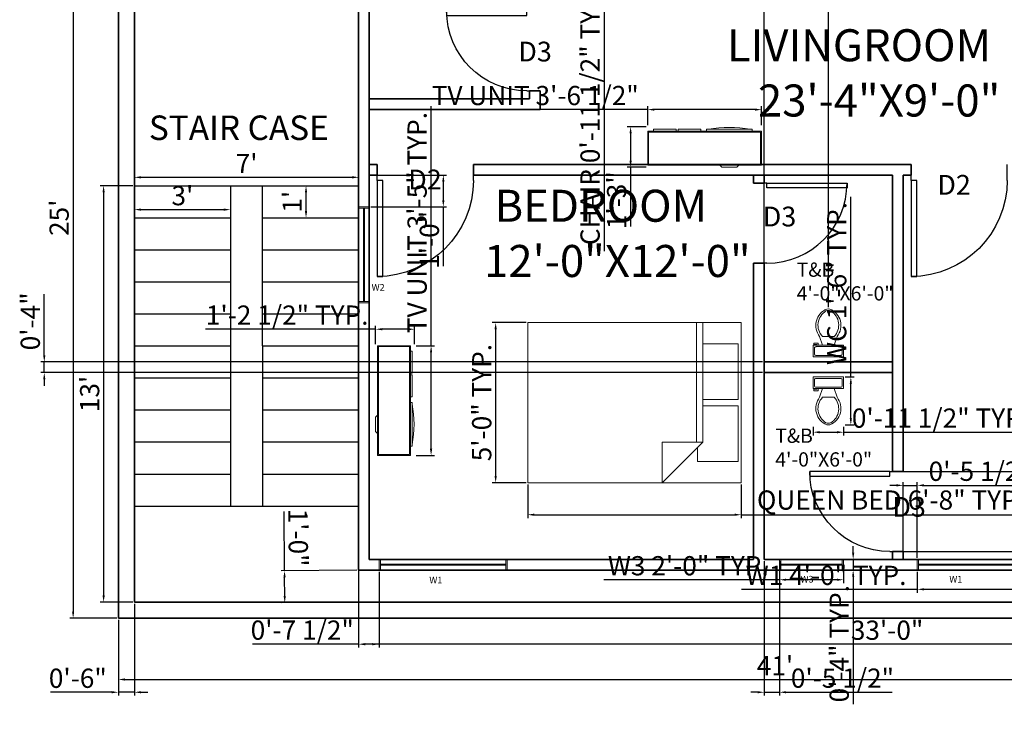
# Model space of a CAD drawing. Units: inches. Extents: x 2165 to 6441, y 2023 to 4425.
# Tile 1 of 4: x 2165 to 2534, y 2023 to 2281. Entities that reach past the tile are written whole.
import ezdxf

# ---------------------------------------------------------------- set-up
doc = ezdxf.new("R2010")
doc.units = ezdxf.units.IN
for name, color, linetype, lineweight in [('A-ANNO-DIMS', 7, 'Continuous', 18), ('A-ANNO-TEXT', 1, 'Continuous', 18), ('A-AREA-IDEN', 1, 'Continuous', 25), ('A-FLOR-FIXT', 9, 'Continuous', 18), ('C-PROP', 7, 'Continuous', 35), ('doors', 5, 'Continuous', 25), ('furniture', 9, 'Continuous', 18), ('stair case', 6, 'Continuous', 25), ('walls', 7, 'Continuous', 35), ('windows', 72, 'Continuous', 18)]:
    doc.layers.add(name, color=color, linetype=linetype, lineweight=lineweight)
doc.styles.get("Standard").update_dxf_attribs({"font": 'arial.ttf'})
doc.dimstyles.new('ISO-25', dxfattribs={"dimtxt": 7.203125, "dimasz": 2.5, "dimexe": 1.25, "dimexo": 0.625, "dimtad": 1, "dimdec": 0, "dimlunit": 4, "dimtxsty": 'Standard', "dimcen": 2.5, "dimadec": 0, "dimazin": 0, "dimtfac": 1, "dimtdec": 0, "dimtmove": 0, "dimatfit": 3, "dimfxl": 1, "dimarcsym": 0})

# ---------------------------------------------------------------- blocks, each defined once
blk = doc.blocks.new('*U2')
for p, q in [((0, 0), (0, -5)), ((30, 0), (30, -5))]:
    blk.add_line(p, q)
blk.add_lwpolyline([(0, 0), (0, 30), (1.75, 30), (1.75, 0)], close=True)
blk.add_arc((0, 0), 30, 0, 90)
blk = doc.blocks.new('Bed - Queen')
for p, q in [((0, -80.00003), (0, 0)), ((0, 0), (59.99999, 0)), ((59.99999, 0), (59.99999, -80.00003)), ((7.99999, -1.2), (28.79998, -1.2)), ((7.99999, -14.4), (7.99999, -1.2)), ((28.79998, -1.2), (28.79998, -14.4)), ((31.19999, -1.2), (51.99999, -1.2)), ((31.19999, -14.4), (31.19999, -1.2)), ((51.99999, -1.2), (51.99999, -16.4)), ((0, -14.4), (44.8, -14.4)), ((59.99999, -29.6), (44.8, -14.4)), ((44.8, -14.4), (44.8, -29.6)), ((44.8, -16.8), (0, -16.8)), ((51.99999, -16.4), (46.79936, -16.4)), ((44.8, -29.6), (59.99999, -29.6)), ((59.99999, -80.00003), (0, -80.00003))]:
    blk.add_line(p, q)
blk = doc.blocks.new('Entertainment Center')
for p, q in [((-4, 0), (-5, -1)), ((4, 0), (-4, 0)), ((5, -1), (4, 0)), ((-17, -19), (-17, -1)), ((-17, -1), (43, -1)), ((-16.5, -18.5), (-16.5, -1.5)), ((-16.5, -1.5), (42.5, -1.5)), ((42.5, -1.5), (42.5, -18.5)), ((43, -1), (43, -19)), ((43, -19), (-17, -19)), ((42.5, -18.5), (-16.5, -18.5)), ((-12, -20), (-12, -19)), ((12, -20), (-12, -20)), ((12, -19), (12, -20)), ((15, -20), (15, -19)), ((27, -20), (15, -20)), ((27, -19), (27, -20)), ((28, -20), (28, -19)), ((40, -20), (28, -20)), ((40, -19), (40, -20))]:
    blk.add_line(p, q)
blk.add_arc((0, 40), 61, 259.6111, 280.3889)
blk = doc.blocks.new('Toilet - top')
for p, q in [((9.5, -6), (9.5, -2)), ((-10, -8.5), (-8, -8.5)), ((-10, -9.5), (-10, -8.5)), ((-7, -9.5), (-10, -9.5)), ((-8, -8.5), (-8, -8)), ((-7, -8), (-7, -9.5)), ((-4, -8), (-6, -14)), ((4, -8), (6, -14)), ((4, -14), (-4, -14))]:
    blk.add_line(p, q)
blk.add_lwpolyline([(10.5, -8), (10.5, 0), (-10.5, 0), (-10.5, -8)], close=True)
for points in [[(-9.5, -2), (-9.5, -6)], [(8.5, -1), (-8.5, -1)], [(-8.5, -7), (8.5, -7)]]:
    blk.add_lwpolyline(points)
for centre, radius, start, end in [((-8.62, -1.88), 0.884, 81.8699, 188.1301), ((-8.62, -6.12), 0.884, 171.8699, 278.1301), ((8.62, -1.88), 0.884, 351.8699, 98.1301), ((8.62, -6.12), 0.884, 261.8699, 8.1301), ((3.52, -21.58), 12.17, 141.46911, 247.97143), ((4.2, -21.82), 11.33, 136.36773, 238.94682), ((-3.52, -21.58), 12.17, 292.02843, 38.53071), ((-4.2, -21.82), 11.33, 301.05301, 43.63209), ((0, -27.88), 4, 245.73182, 294.26817), ((0, -29), 4, 254.86053, 285.13947)]:
    blk.add_arc(centre, radius, start, end)
blk = doc.blocks.new('*D10')
at = {"layer": 'A-ANNO-DIMS', "color": 0, "lineweight": -2, "transparency": 16777216}
for p, q in [((2201.06, 2356.78), (2183.49, 2356.78)), ((2184.74, 2354.28), (2184.74, 2059.28)), ((2201.06, 2056.78), (2183.49, 2056.78))]:
    blk.add_line(p, q, dxfattribs=at)
at = {"layer": 'A-ANNO-DIMS', "color": 0, "transparency": 16777216}
for points in [[(2184.32, 2354.28), (2185.15, 2354.28), (2184.74, 2356.78)], [(2184.32, 2059.28), (2185.15, 2059.28), (2184.74, 2056.78)]]:
    blk.add_solid(points, dxfattribs=at)
at = {"layer": 'Defpoints', "color": 0, "transparency": 16777216}
for p in [(2201.68, 2356.78), (2184.74, 2056.78), (2201.68, 2056.78)]:
    blk.add_point(p, dxfattribs=at)
at = {"layer": 'A-ANNO-DIMS', "color": 0, "transparency": 16777216, "insert": (2180.43, 2206.78), "char_height": 7.203, "attachment_point": 5, "rotation": 90}
blk.add_mtext("25'", dxfattribs=at)
blk = doc.blocks.new('*D11')
at = {"layer": 'A-ANNO-DIMS', "color": 0, "lineweight": -2, "transparency": 16777216}
for p, q in [((2201.68, 2056.16), (2201.68, 2032.56)), ((2693.68, 2056.16), (2693.68, 2032.56)), ((2204.18, 2033.81), (2691.18, 2033.81))]:
    blk.add_line(p, q, dxfattribs=at)
at = {"layer": 'A-ANNO-DIMS', "color": 0, "transparency": 16777216}
for points in [[(2204.18, 2034.23), (2204.18, 2033.39), (2201.68, 2033.81)], [(2691.18, 2034.23), (2691.18, 2033.39), (2693.68, 2033.81)]]:
    blk.add_solid(points, dxfattribs=at)
at = {"layer": 'Defpoints', "color": 0, "transparency": 16777216}
for p in [(2201.68, 2056.78), (2693.68, 2056.78), (2693.68, 2033.81)]:
    blk.add_point(p, dxfattribs=at)
at = {"layer": 'A-ANNO-DIMS', "color": 0, "transparency": 16777216, "insert": (2447.68, 2038.05), "char_height": 7.203, "attachment_point": 5}
blk.add_mtext("41'", dxfattribs=at)
blk = doc.blocks.new('*D12')
at = {"layer": 'A-ANNO-DIMS', "color": 0, "lineweight": -2, "transparency": 16777216}
for p, q in [((2207.68, 2218.16), (2207.68, 2208.58)), ((2243.68, 2218.16), (2243.68, 2208.58)), ((2210.18, 2209.83), (2241.18, 2209.83))]:
    blk.add_line(p, q, dxfattribs=at)
at = {"layer": 'A-ANNO-DIMS', "color": 0, "transparency": 16777216}
for points in [[(2210.18, 2210.25), (2210.18, 2209.41), (2207.68, 2209.83)], [(2241.18, 2210.25), (2241.18, 2209.41), (2243.68, 2209.83)]]:
    blk.add_solid(points, dxfattribs=at)
at = {"layer": 'Defpoints', "color": 0, "transparency": 16777216}
for p in [(2207.68, 2218.78), (2243.68, 2218.78), (2243.68, 2209.83)]:
    blk.add_point(p, dxfattribs=at)
at = {"layer": 'A-ANNO-DIMS', "color": 0, "transparency": 16777216, "insert": (2225.68, 2214.13), "char_height": 7.203, "attachment_point": 5}
blk.add_mtext("3'", dxfattribs=at)
blk = doc.blocks.new('*D13')
at = {"layer": 'A-ANNO-DIMS', "color": 0, "lineweight": -2, "transparency": 16777216}
for p, q in [((2256.31, 2218.78), (2273.24, 2218.78)), ((2271.99, 2209.28), (2271.99, 2216.28)), ((2256.32, 2206.78), (2273.24, 2206.78))]:
    blk.add_line(p, q, dxfattribs=at)
at = {"layer": 'A-ANNO-DIMS', "color": 0, "transparency": 16777216}
for points in [[(2271.58, 2216.28), (2272.41, 2216.28), (2271.99, 2218.78)], [(2271.58, 2209.28), (2272.41, 2209.28), (2271.99, 2206.78)]]:
    blk.add_solid(points, dxfattribs=at)
at = {"layer": 'Defpoints', "color": 0, "transparency": 16777216}
for p in [(2255.69, 2218.78), (2271.99, 2218.78), (2255.69, 2206.78)]:
    blk.add_point(p, dxfattribs=at)
at = {"layer": 'A-ANNO-DIMS', "color": 0, "transparency": 16777216, "insert": (2267.75, 2212.78), "char_height": 7.203, "attachment_point": 5, "rotation": 90}
blk.add_mtext("1'", dxfattribs=at)
blk = doc.blocks.new('*D14')
at = {"layer": 'A-ANNO-DIMS', "color": 0, "lineweight": -2, "transparency": 16777216}
for p, q in [((2207.68, 2219.41), (2207.68, 2223.18)), ((2210.18, 2221.93), (2289.28, 2221.93)), ((2291.78, 2219.41), (2291.78, 2223.18))]:
    blk.add_line(p, q, dxfattribs=at)
at = {"layer": 'A-ANNO-DIMS', "color": 0, "transparency": 16777216}
for points in [[(2210.18, 2222.35), (2210.18, 2221.52), (2207.68, 2221.93)], [(2289.28, 2222.35), (2289.28, 2221.52), (2291.78, 2221.93)]]:
    blk.add_solid(points, dxfattribs=at)
at = {"layer": 'Defpoints', "color": 0, "transparency": 16777216}
for p in [(2291.78, 2221.93), (2207.68, 2218.78), (2291.78, 2218.78)]:
    blk.add_point(p, dxfattribs=at)
at = {"layer": 'A-ANNO-DIMS', "color": 0, "transparency": 16777216, "insert": (2249.73, 2226.16), "char_height": 7.203, "attachment_point": 5}
blk.add_mtext("7'", dxfattribs=at)
blk = doc.blocks.new('*D22')
at = {"layer": 'A-ANNO-DIMS', "color": 0, "lineweight": -2, "transparency": 16777216}
for p, q in [((2207.06, 2218.78), (2194.91, 2218.78)), ((2196.16, 2216.28), (2196.16, 2065.28)), ((2207.06, 2062.78), (2194.91, 2062.78))]:
    blk.add_line(p, q, dxfattribs=at)
at = {"layer": 'A-ANNO-DIMS', "color": 0, "transparency": 16777216}
for points in [[(2195.75, 2216.28), (2196.58, 2216.28), (2196.16, 2218.78)], [(2195.75, 2065.28), (2196.58, 2065.28), (2196.16, 2062.78)]]:
    blk.add_solid(points, dxfattribs=at)
at = {"layer": 'Defpoints', "color": 0, "transparency": 16777216}
for p in [(2207.68, 2218.78), (2196.16, 2062.78), (2207.68, 2062.78)]:
    blk.add_point(p, dxfattribs=at)
at = {"layer": 'A-ANNO-DIMS', "color": 0, "transparency": 16777216, "insert": (2191.86, 2140.78), "char_height": 7.203, "attachment_point": 5, "rotation": 90}
blk.add_mtext("13'", dxfattribs=at)
blk = doc.blocks.new('WIN-W2-36IN')
for p, q in [((0, 4), (36, 4)), ((0, 0), (0, 4)), ((0.5, 0), (0.5, 4)), ((35.5, 4), (35.5, 0)), ((36, 4), (36, 0)), ((36, 0), (0, 0)), ((0.5, 2.2), (35.5, 2.2)), ((0.5, 1.8), (35.5, 1.8)), ((0.5, 1.8), (35.5, 1.8))]:
    blk.add_line(p, q)
blk = doc.blocks.new('WIN-W1-48IN')
for p, q in [((0, 4), (48, 4)), ((0, 0), (0, 4)), ((0.5, 0), (0.5, 4)), ((47.5, 4), (47.5, 0)), ((48, 4), (48, 0)), ((48, 0), (0, 0)), ((0.5, 2.2), (47.5, 2.2)), ((0.5, 1.8), (47.5, 1.8))]:
    blk.add_line(p, q)
blk = doc.blocks.new('WIN-W3-24IN')
for p, q in [((0, 4), (24, 4)), ((0, 0), (0, 4)), ((0.5, 0), (0.5, 4)), ((23.5, 0), (23.5, 4)), ((24, 0), (24, 4)), ((24, 0), (0, 0)), ((23.5, 2.2), (0.5, 2.2)), ((23.5, 1.8), (0.5, 1.8))]:
    blk.add_line(p, q)
blk = doc.blocks.new('*D26')
at = {"layer": 'A-ANNO-DIMS', "color": 0, "lineweight": -2, "transparency": 16777216}
for p, q in [((2500.99, 2074.16), (2500.99, 2066.33)), ((2549, 2074.16), (2549, 2066.33)), ((2500.99, 2067.58), (2435.15, 2067.58)), ((2546.5, 2067.58), (2503.49, 2067.58))]:
    blk.add_line(p, q, dxfattribs=at)
at = {"layer": 'A-ANNO-DIMS', "color": 0, "transparency": 16777216}
for points in [[(2503.49, 2068), (2503.49, 2067.17), (2500.99, 2067.58)], [(2546.5, 2068), (2546.5, 2067.17), (2549, 2067.58)]]:
    blk.add_solid(points, dxfattribs=at)
at = {"layer": 'Defpoints', "color": 0, "transparency": 16777216}
for p in [(2500.99, 2074.78), (2549, 2074.78), (2500.99, 2067.58)]:
    blk.add_point(p, dxfattribs=at)
at = {"layer": 'A-ANNO-DIMS', "color": 0, "transparency": 16777216, "insert": (2466.82, 2071.89), "char_height": 7.2031, "attachment_point": 5}
blk.add_mtext('W1 4\'-0" TYP.', dxfattribs=at)
blk = doc.blocks.new('*D30')
at = {"layer": 'A-ANNO-DIMS', "color": 0, "lineweight": -2, "transparency": 16777216}
for p, q in [((2449.37, 2074.16), (2449.37, 2069.93)), ((2473.37, 2074.16), (2473.37, 2069.93)), ((2449.37, 2071.18), (2383.53, 2071.18)), ((2470.87, 2071.18), (2451.87, 2071.18))]:
    blk.add_line(p, q, dxfattribs=at)
at = {"layer": 'A-ANNO-DIMS', "color": 0, "transparency": 16777216}
for points in [[(2451.87, 2071.6), (2451.87, 2070.77), (2449.37, 2071.18)], [(2470.87, 2071.6), (2470.87, 2070.77), (2473.37, 2071.18)]]:
    blk.add_solid(points, dxfattribs=at)
at = {"layer": 'Defpoints', "color": 0, "transparency": 16777216}
for p in [(2449.37, 2074.78), (2473.37, 2074.78), (2449.37, 2071.18)]:
    blk.add_point(p, dxfattribs=at)
at = {"layer": 'A-ANNO-DIMS', "color": 0, "transparency": 16777216, "insert": (2415.2, 2075.49), "char_height": 7.2031, "attachment_point": 5}
blk.add_mtext('W3 2\'-0" TYP.', dxfattribs=at)
blk = doc.blocks.new('*D31')
at = {"layer": 'A-ANNO-DIMS', "color": 0, "lineweight": -2, "transparency": 16777216}
for p, q in [((2476.97, 2081.28), (2476.97, 2083.78)), ((2474, 2078.78), (2478.22, 2078.78)), ((2476.97, 2078.78), (2476.97, 2074.78)), ((2474, 2074.78), (2478.22, 2074.78)), ((2476.97, 2072.28), (2476.97, 2024.63))]:
    blk.add_line(p, q, dxfattribs=at)
at = {"layer": 'A-ANNO-DIMS', "color": 0, "transparency": 16777216}
for points in [[(2476.56, 2081.28), (2477.39, 2081.28), (2476.97, 2078.78)], [(2476.56, 2072.28), (2477.39, 2072.28), (2476.97, 2074.78)]]:
    blk.add_solid(points, dxfattribs=at)
at = {"layer": 'Defpoints', "color": 0, "transparency": 16777216}
for p in [(2473.37, 2078.78), (2473.37, 2074.78), (2476.97, 2074.78)]:
    blk.add_point(p, dxfattribs=at)
at = {"layer": 'A-ANNO-DIMS', "color": 0, "transparency": 16777216, "insert": (2472.67, 2047.21), "char_height": 7.203, "attachment_point": 5, "rotation": 90}
blk.add_mtext('0\'-4" TYP.', dxfattribs=at)
blk = doc.blocks.new('*D32')
at = {"layer": 'A-ANNO-DIMS', "color": 0, "lineweight": -2, "transparency": 16777216}
for p, q in [((2355.04, 2106.91), (2355.04, 2094.28)), ((2435.04, 2106.91), (2435.04, 2094.28)), ((2357.54, 2095.53), (2432.54, 2095.53)), ((2435.04, 2095.53), (2544.75, 2095.53))]:
    blk.add_line(p, q, dxfattribs=at)
at = {"layer": 'A-ANNO-DIMS', "color": 0, "transparency": 16777216}
for points in [[(2357.54, 2095.95), (2357.54, 2095.11), (2355.04, 2095.53)], [(2432.54, 2095.95), (2432.54, 2095.11), (2435.04, 2095.53)]]:
    blk.add_solid(points, dxfattribs=at)
at = {"layer": 'Defpoints', "color": 0, "transparency": 16777216}
for p in [(2355.04, 2107.53), (2435.04, 2107.53), (2435.04, 2095.53)]:
    blk.add_point(p, dxfattribs=at)
at = {"layer": 'A-ANNO-DIMS', "color": 0, "transparency": 16777216, "insert": (2491.14, 2100.1), "char_height": 7.2031, "attachment_point": 5}
blk.add_mtext('QUEEN BED 6\'-8" TYP.', dxfattribs=at)
blk = doc.blocks.new('*D33')
at = {"layer": 'A-ANNO-DIMS', "color": 0, "lineweight": -2, "transparency": 16777216}
for p, q in [((2354.41, 2167.53), (2341.79, 2167.53)), ((2343.04, 2165.03), (2343.04, 2110.03)), ((2354.41, 2107.53), (2341.79, 2107.53))]:
    blk.add_line(p, q, dxfattribs=at)
at = {"layer": 'A-ANNO-DIMS', "color": 0, "transparency": 16777216}
for points in [[(2342.62, 2165.03), (2343.45, 2165.03), (2343.04, 2167.53)], [(2342.62, 2110.03), (2343.45, 2110.03), (2343.04, 2107.53)]]:
    blk.add_solid(points, dxfattribs=at)
at = {"layer": 'Defpoints', "color": 0, "transparency": 16777216}
for p in [(2355.04, 2167.53), (2343.04, 2107.53), (2355.04, 2107.53)]:
    blk.add_point(p, dxfattribs=at)
at = {"layer": 'A-ANNO-DIMS', "color": 0, "transparency": 16777216, "insert": (2338.74, 2137.53), "char_height": 7.203, "attachment_point": 5, "rotation": 90}
blk.add_mtext('5\'-0" TYP.', dxfattribs=at)
blk = doc.blocks.new('*D34')
at = {"layer": 'A-ANNO-DIMS', "color": 0, "lineweight": -2, "transparency": 16777216}
for p, q in [((2384.79, 2309.82), (2382.44, 2309.82)), ((2383.69, 2307.32), (2383.69, 2300.85)), ((2384.79, 2298.35), (2382.44, 2298.35)), ((2383.69, 2298.35), (2383.69, 2194.29))]:
    blk.add_line(p, q, dxfattribs=at)
at = {"layer": 'A-ANNO-DIMS', "color": 0, "transparency": 16777216}
for points in [[(2383.27, 2307.32), (2384.11, 2307.32), (2383.69, 2309.82)], [(2383.27, 2300.85), (2384.11, 2300.85), (2383.69, 2298.35)]]:
    blk.add_solid(points, dxfattribs=at)
at = {"layer": 'Defpoints', "color": 0, "transparency": 16777216}
for p in [(2385.41, 2309.82), (2383.69, 2298.35), (2385.41, 2298.35)]:
    blk.add_point(p, dxfattribs=at)
at = {"layer": 'A-ANNO-DIMS', "color": 0, "transparency": 16777216, "insert": (2379.34, 2245.07), "char_height": 7.2031, "attachment_point": 5, "rotation": 90}
blk.add_mtext('CHAIR 0\'-11 1/2" TYP.', dxfattribs=at)
blk = doc.blocks.new('*D36')
at = {"layer": 'A-ANNO-DIMS', "color": 0, "lineweight": -2, "transparency": 16777216}
for p, q in [((2400, 2247.29), (2318.21, 2247.29)), ((2400, 2241.51), (2400, 2248.54)), ((2440.17, 2247.29), (2402.5, 2247.29)), ((2442.67, 2241.51), (2442.67, 2248.54))]:
    blk.add_line(p, q, dxfattribs=at)
at = {"layer": 'A-ANNO-DIMS', "color": 0, "transparency": 16777216}
for points in [[(2402.5, 2247.71), (2402.5, 2246.87), (2400, 2247.29)], [(2440.17, 2247.71), (2440.17, 2246.87), (2442.67, 2247.29)]]:
    blk.add_solid(points, dxfattribs=at)
at = {"layer": 'Defpoints', "color": 0, "transparency": 16777216}
for p in [(2400, 2247.29), (2400, 2240.89), (2442.67, 2240.89)]:
    blk.add_point(p, dxfattribs=at)
at = {"layer": 'A-ANNO-DIMS', "color": 0, "transparency": 16777216, "insert": (2357.86, 2251.64), "char_height": 7.2031, "attachment_point": 5}
blk.add_mtext('TV UNIT 3\'-6 1/2"', dxfattribs=at)
blk = doc.blocks.new('*D37')
at = {"layer": 'A-ANNO-DIMS', "color": 0, "lineweight": -2, "transparency": 16777216}
for p, q in [((2399.38, 2240.89), (2392.35, 2240.89)), ((2393.6, 2238.39), (2393.6, 2228.22)), ((2399.38, 2225.72), (2392.35, 2225.72)), ((2393.6, 2225.72), (2393.6, 2203.5))]:
    blk.add_line(p, q, dxfattribs=at)
at = {"layer": 'A-ANNO-DIMS', "color": 0, "transparency": 16777216}
for points in [[(2393.18, 2238.39), (2394.02, 2238.39), (2393.6, 2240.89)], [(2393.18, 2228.22), (2394.02, 2228.22), (2393.6, 2225.72)]]:
    blk.add_solid(points, dxfattribs=at)
at = {"layer": 'Defpoints', "color": 0, "transparency": 16777216}
for p in [(2400, 2240.89), (2393.6, 2225.72), (2400, 2225.72)]:
    blk.add_point(p, dxfattribs=at)
at = {"layer": 'A-ANNO-DIMS', "color": 0, "transparency": 16777216, "insert": (2389.3, 2213.36), "char_height": 7.203, "attachment_point": 5, "rotation": 90}
blk.add_mtext('1\'-3"', dxfattribs=at)
blk = doc.blocks.new('*D38')
at = {"layer": 'A-ANNO-DIMS', "color": 0, "lineweight": -2, "transparency": 16777216}
for p, q in [((2318.85, 2158.86), (2318.85, 2248.63)), ((2313.31, 2158.86), (2320.1, 2158.86)), ((2318.85, 2120.25), (2318.85, 2156.36)), ((2313.31, 2117.75), (2320.1, 2117.75))]:
    blk.add_line(p, q, dxfattribs=at)
at = {"layer": 'A-ANNO-DIMS', "color": 0, "transparency": 16777216}
for points in [[(2318.43, 2156.36), (2319.26, 2156.36), (2318.85, 2158.86)], [(2318.43, 2120.25), (2319.26, 2120.25), (2318.85, 2117.75)]]:
    blk.add_solid(points, dxfattribs=at)
at = {"layer": 'Defpoints', "color": 0, "transparency": 16777216}
for p in [(2312.68, 2158.86), (2318.85, 2158.86), (2312.68, 2117.75)]:
    blk.add_point(p, dxfattribs=at)
at = {"layer": 'A-ANNO-DIMS', "color": 0, "transparency": 16777216, "insert": (2314.54, 2204.99), "char_height": 7.2031, "attachment_point": 5, "rotation": 90}
blk.add_mtext('TV UNIT 3\'-5" TYP.', dxfattribs=at)
blk = doc.blocks.new('*D39')
at = {"layer": 'A-ANNO-DIMS', "color": 0, "lineweight": -2, "transparency": 16777216}
for p, q in [((2298.06, 2159.49), (2298.06, 2166.28)), ((2312.68, 2159.49), (2312.68, 2166.28)), ((2298.06, 2165.03), (2234.3, 2165.03)), ((2310.18, 2165.03), (2300.56, 2165.03))]:
    blk.add_line(p, q, dxfattribs=at)
at = {"layer": 'A-ANNO-DIMS', "color": 0, "transparency": 16777216}
for points in [[(2300.56, 2165.44), (2300.56, 2164.61), (2298.06, 2165.03)], [(2310.18, 2165.44), (2310.18, 2164.61), (2312.68, 2165.03)]]:
    blk.add_solid(points, dxfattribs=at)
at = {"layer": 'Defpoints', "color": 0, "transparency": 16777216}
for p in [(2298.06, 2165.03), (2298.06, 2158.86), (2312.68, 2158.86)]:
    blk.add_point(p, dxfattribs=at)
at = {"layer": 'A-ANNO-DIMS', "color": 0, "transparency": 16777216, "insert": (2264.93, 2169.38), "char_height": 7.2031, "attachment_point": 5}
blk.add_mtext('1\'-2 1/2" TYP.', dxfattribs=at)
blk = doc.blocks.new('*D42')
at = {"layer": 'A-ANNO-DIMS', "color": 0, "lineweight": -2, "transparency": 16777216}
for p, q in [((2476.1, 2147.15), (2476.1, 2214.66)), ((2474.03, 2147.15), (2477.35, 2147.15)), ((2476.1, 2131.65), (2476.1, 2144.65)), ((2474.03, 2129.15), (2477.35, 2129.15))]:
    blk.add_line(p, q, dxfattribs=at)
at = {"layer": 'A-ANNO-DIMS', "color": 0, "transparency": 16777216}
for points in [[(2475.69, 2144.65), (2476.52, 2144.65), (2476.1, 2147.15)], [(2475.69, 2131.65), (2476.52, 2131.65), (2476.1, 2129.15)]]:
    blk.add_solid(points, dxfattribs=at)
at = {"layer": 'Defpoints', "color": 0, "transparency": 16777216}
for p in [(2473.4, 2147.15), (2476.1, 2147.15), (2473.4, 2129.15)]:
    blk.add_point(p, dxfattribs=at)
at = {"layer": 'A-ANNO-DIMS', "color": 0, "transparency": 16777216, "insert": (2471.76, 2182.16), "char_height": 7.2031, "attachment_point": 5, "rotation": 90}
blk.add_mtext('WC 1\'-6" TYP.', dxfattribs=at)
blk = doc.blocks.new('*D43')
at = {"layer": 'A-ANNO-DIMS', "color": 0, "lineweight": -2, "transparency": 16777216}
for p, q in [((2461.96, 2128.52), (2461.96, 2125.2)), ((2473.4, 2128.52), (2473.4, 2125.2)), ((2464.46, 2126.45), (2470.9, 2126.45)), ((2473.4, 2126.45), (2543.44, 2126.45))]:
    blk.add_line(p, q, dxfattribs=at)
at = {"layer": 'A-ANNO-DIMS', "color": 0, "transparency": 16777216}
for points in [[(2464.46, 2126.86), (2464.46, 2126.03), (2461.96, 2126.45)], [(2470.9, 2126.86), (2470.9, 2126.03), (2473.4, 2126.45)]]:
    blk.add_solid(points, dxfattribs=at)
at = {"layer": 'Defpoints', "color": 0, "transparency": 16777216}
for p in [(2461.96, 2129.15), (2473.4, 2129.15), (2473.4, 2126.45)]:
    blk.add_point(p, dxfattribs=at)
at = {"layer": 'A-ANNO-DIMS', "color": 0, "transparency": 16777216, "insert": (2509.67, 2130.8), "char_height": 7.2031, "attachment_point": 5}
blk.add_mtext('0\'-11 1/2" TYP.', dxfattribs=at)
blk = doc.blocks.new('*D48')
at = {"layer": 'A-ANNO-DIMS', "color": 0, "lineweight": -2, "transparency": 16777216}
for p, q in [((2492.31, 2111.78), (2722.68, 2111.78)), ((2721.43, 2084.28), (2721.43, 2109.28)), ((2492.31, 2081.78), (2722.68, 2081.78))]:
    blk.add_line(p, q, dxfattribs=at)
at = {"layer": 'A-ANNO-DIMS', "color": 0, "transparency": 16777216}
for points in [[(2721.02, 2109.28), (2721.85, 2109.28), (2721.43, 2111.78)], [(2721.02, 2084.28), (2721.85, 2084.28), (2721.43, 2081.78)]]:
    blk.add_solid(points, dxfattribs=at)
at = {"layer": 'Defpoints', "color": 0, "transparency": 16777216}
for p in [(2491.68, 2111.78), (2721.43, 2111.78), (2491.68, 2081.78)]:
    blk.add_point(p, dxfattribs=at)
at = {"layer": 'A-ANNO-DIMS', "color": 0, "transparency": 16777216, "insert": (2717.13, 2096.78), "char_height": 7.203, "attachment_point": 5, "rotation": 90}
blk.add_mtext('2\'-6"', dxfattribs=at)
blk = doc.blocks.new('*D49')
at = {"layer": 'A-ANNO-DIMS', "color": 0, "lineweight": -2, "transparency": 16777216}
for p, q in [((2207.68, 2062.16), (2207.68, 2027.78)), ((2201.68, 2056.16), (2201.68, 2027.78)), ((2199.18, 2029.03), (2176.29, 2029.03)), ((2207.68, 2029.03), (2201.68, 2029.03)), ((2210.18, 2029.03), (2212.68, 2029.03))]:
    blk.add_line(p, q, dxfattribs=at)
at = {"layer": 'A-ANNO-DIMS', "color": 0, "transparency": 16777216}
for points in [[(2199.18, 2029.45), (2199.18, 2028.62), (2201.68, 2029.03)], [(2210.18, 2029.45), (2210.18, 2028.62), (2207.68, 2029.03)]]:
    blk.add_solid(points, dxfattribs=at)
at = {"layer": 'Defpoints', "color": 0, "transparency": 16777216}
for p in [(2207.68, 2062.78), (2201.68, 2056.78), (2201.68, 2029.03)]:
    blk.add_point(p, dxfattribs=at)
at = {"layer": 'A-ANNO-DIMS', "color": 0, "transparency": 16777216, "insert": (2186.49, 2033.34), "char_height": 7.203, "attachment_point": 5}
blk.add_mtext('0\'-6"', dxfattribs=at)
blk = doc.blocks.new('*D50')
at = {"layer": 'A-ANNO-DIMS', "color": 0, "lineweight": -2, "transparency": 16777216}
for p, q in [((2263.93, 2074.56), (2263.76, 2096.78)), ((2291.06, 2074.78), (2262.68, 2074.55)), ((2264.01, 2065.06), (2263.95, 2072.06)), ((2291.15, 2062.78), (2262.78, 2062.55))]:
    blk.add_line(p, q, dxfattribs=at)
at = {"layer": 'A-ANNO-DIMS', "color": 0, "transparency": 16777216}
for points in [[(2264.37, 2072.07), (2263.54, 2072.06), (2263.93, 2074.56)], [(2264.43, 2065.07), (2263.59, 2065.06), (2264.03, 2062.56)]]:
    blk.add_solid(points, dxfattribs=at)
at = {"layer": 'Defpoints', "color": 0, "transparency": 16777216}
for p in [(2263.93, 2074.56), (2291.68, 2074.78), (2291.78, 2062.78)]:
    blk.add_point(p, dxfattribs=at)
at = {"layer": 'A-ANNO-DIMS', "color": 0, "transparency": 16777216, "insert": (2268.14, 2086.96), "char_height": 7.203, "attachment_point": 5, "rotation": 270.4537}
blk.add_mtext('1\'-0"', dxfattribs=at)
blk = doc.blocks.new('*D51')
at = {"layer": 'A-ANNO-DIMS', "color": 0, "lineweight": -2, "transparency": 16777216}
for p, q in [((2291.68, 2074.16), (2291.68, 2045.78)), ((2687.68, 2074.16), (2687.68, 2045.78)), ((2685.18, 2047.03), (2294.18, 2047.03))]:
    blk.add_line(p, q, dxfattribs=at)
at = {"layer": 'A-ANNO-DIMS', "color": 0, "transparency": 16777216}
for points in [[(2294.18, 2047.45), (2294.18, 2046.62), (2291.68, 2047.03)], [(2685.18, 2047.45), (2685.18, 2046.62), (2687.68, 2047.03)]]:
    blk.add_solid(points, dxfattribs=at)
at = {"layer": 'Defpoints', "color": 0, "transparency": 16777216}
for p in [(2291.68, 2074.78), (2687.68, 2074.78), (2291.68, 2047.03)]:
    blk.add_point(p, dxfattribs=at)
at = {"layer": 'A-ANNO-DIMS', "color": 0, "transparency": 16777216, "insert": (2489.68, 2051.34), "char_height": 7.203, "attachment_point": 5}
blk.add_mtext('33\'-0"', dxfattribs=at)
blk = doc.blocks.new('*D53')
at = {"layer": 'A-ANNO-DIMS', "color": 0, "lineweight": -2, "transparency": 16777216}
for p, q in [((2173.93, 2155.28), (2173.93, 2178.18)), ((2443.06, 2152.78), (2172.68, 2152.78)), ((2173.93, 2148.78), (2173.93, 2152.78)), ((2443.06, 2148.78), (2172.68, 2148.78)), ((2173.93, 2146.28), (2173.93, 2143.78))]:
    blk.add_line(p, q, dxfattribs=at)
at = {"layer": 'A-ANNO-DIMS', "color": 0, "transparency": 16777216}
for points in [[(2173.52, 2155.28), (2174.35, 2155.28), (2173.93, 2152.78)], [(2173.52, 2146.28), (2174.35, 2146.28), (2173.93, 2148.78)]]:
    blk.add_solid(points, dxfattribs=at)
at = {"layer": 'Defpoints', "color": 0, "transparency": 16777216}
for p in [(2173.93, 2152.78), (2443.68, 2152.78), (2443.68, 2148.78)]:
    blk.add_point(p, dxfattribs=at)
at = {"layer": 'A-ANNO-DIMS', "color": 0, "transparency": 16777216, "insert": (2169.63, 2167.98), "char_height": 7.203, "attachment_point": 5, "rotation": 90}
blk.add_mtext('0\'-4"', dxfattribs=at)
blk = doc.blocks.new('*D54')
at = {"layer": 'A-ANNO-DIMS', "color": 0, "lineweight": -2, "transparency": 16777216}
for p, q in [((2443.68, 2153.41), (2443.68, 2443.73)), ((2446.18, 2442.48), (2465.18, 2442.48)), ((2467.68, 2173.28), (2467.68, 2443.73))]:
    blk.add_line(p, q, dxfattribs=at)
at = {"layer": 'A-ANNO-DIMS', "color": 0, "transparency": 16777216}
for points in [[(2446.18, 2442.9), (2446.18, 2442.06), (2443.68, 2442.48)], [(2465.18, 2442.9), (2465.18, 2442.06), (2467.68, 2442.48)]]:
    blk.add_solid(points, dxfattribs=at)
at = {"layer": 'Defpoints', "color": 0, "transparency": 16777216}
for p in [(2467.68, 2442.48), (2467.68, 2172.66), (2443.68, 2152.78)]:
    blk.add_point(p, dxfattribs=at)
at = {"layer": 'A-ANNO-DIMS', "color": 0, "transparency": 16777216, "insert": (2455.68, 2446.78), "char_height": 7.203, "attachment_point": 5}
blk.add_mtext('2\'-0"', dxfattribs=at)
blk = doc.blocks.new('*D55')
at = {"layer": 'A-ANNO-DIMS', "color": 0, "lineweight": -2, "transparency": 16777216}
for p, q in [((2443.68, 2078.16), (2443.68, 2027.78)), ((2449.37, 2078.16), (2449.37, 2027.78)), ((2441.18, 2029.03), (2438.68, 2029.03)), ((2443.68, 2029.03), (2449.37, 2029.03)), ((2451.87, 2029.03), (2491.55, 2029.03))]:
    blk.add_line(p, q, dxfattribs=at)
at = {"layer": 'A-ANNO-DIMS', "color": 0, "transparency": 16777216}
for points in [[(2441.18, 2029.45), (2441.18, 2028.62), (2443.68, 2029.03)], [(2451.87, 2029.45), (2451.87, 2028.62), (2449.37, 2029.03)]]:
    blk.add_solid(points, dxfattribs=at)
at = {"layer": 'Defpoints', "color": 0, "transparency": 16777216}
for p in [(2443.68, 2078.78), (2449.37, 2078.78), (2449.37, 2029.03)]:
    blk.add_point(p, dxfattribs=at)
at = {"layer": 'A-ANNO-DIMS', "color": 0, "transparency": 16777216, "insert": (2472.96, 2033.38), "char_height": 7.203, "attachment_point": 5}
blk.add_mtext('0\'-5 1/2"', dxfattribs=at)
blk = doc.blocks.new('*D59')
at = {"layer": 'A-ANNO-DIMS', "color": 0, "lineweight": -2, "transparency": 16777216}
for p, q in [((2291.68, 2074.16), (2291.68, 2045.78)), ((2299.39, 2074.16), (2299.39, 2045.78)), ((2291.68, 2047.03), (2252, 2047.03)), ((2296.89, 2047.03), (2294.18, 2047.03))]:
    blk.add_line(p, q, dxfattribs=at)
at = {"layer": 'A-ANNO-DIMS', "color": 0, "transparency": 16777216}
for points in [[(2294.18, 2047.45), (2294.18, 2046.62), (2291.68, 2047.03)], [(2296.89, 2047.45), (2296.89, 2046.62), (2299.39, 2047.03)]]:
    blk.add_solid(points, dxfattribs=at)
at = {"layer": 'Defpoints', "color": 0, "transparency": 16777216}
for p in [(2291.68, 2074.78), (2299.39, 2074.78), (2291.68, 2047.03)]:
    blk.add_point(p, dxfattribs=at)
at = {"layer": 'A-ANNO-DIMS', "color": 0, "transparency": 16777216, "insert": (2270.59, 2051.38), "char_height": 7.203, "attachment_point": 5}
blk.add_mtext('0\'-7 1/2"', dxfattribs=at)
blk = doc.blocks.new('*D60')
at = {"layer": 'A-ANNO-DIMS', "color": 0, "lineweight": -2, "transparency": 16777216}
for p, q in [((2493.18, 2106.53), (2490.68, 2106.53)), ((2495.68, 2079.41), (2495.68, 2107.78)), ((2495.68, 2106.53), (2500.99, 2106.53)), ((2500.99, 2079.41), (2500.99, 2107.78)), ((2503.49, 2106.53), (2543.17, 2106.53))]:
    blk.add_line(p, q, dxfattribs=at)
at = {"layer": 'A-ANNO-DIMS', "color": 0, "transparency": 16777216}
for points in [[(2493.18, 2106.95), (2493.18, 2106.12), (2495.68, 2106.53)], [(2503.49, 2106.95), (2503.49, 2106.12), (2500.99, 2106.53)]]:
    blk.add_solid(points, dxfattribs=at)
at = {"layer": 'Defpoints', "color": 0, "transparency": 16777216}
for p in [(2500.99, 2106.53), (2495.68, 2078.78), (2500.99, 2078.78)]:
    blk.add_point(p, dxfattribs=at)
at = {"layer": 'A-ANNO-DIMS', "color": 0, "transparency": 16777216, "insert": (2524.58, 2110.88), "char_height": 7.203, "attachment_point": 5}
blk.add_mtext('0\'-5 1/2"', dxfattribs=at)
blk = doc.blocks.new('*D62')
at = {"layer": 'A-ANNO-DIMS', "color": 0, "lineweight": -2, "transparency": 16777216}
for p, q in [((2296.31, 2222.78), (2324.68, 2222.78)), ((2323.43, 2220.28), (2323.43, 2213.36)), ((2296.31, 2210.86), (2324.68, 2210.86)), ((2323.43, 2210.86), (2323.43, 2188.64))]:
    blk.add_line(p, q, dxfattribs=at)
at = {"layer": 'A-ANNO-DIMS', "color": 0, "transparency": 16777216}
for points in [[(2323.02, 2220.28), (2323.85, 2220.28), (2323.43, 2222.78)], [(2323.02, 2213.36), (2323.85, 2213.36), (2323.43, 2210.86)]]:
    blk.add_solid(points, dxfattribs=at)
at = {"layer": 'Defpoints', "color": 0, "transparency": 16777216}
for p in [(2295.68, 2222.78), (2295.68, 2210.86), (2323.43, 2210.86)]:
    blk.add_point(p, dxfattribs=at)
at = {"layer": 'A-ANNO-DIMS', "color": 0, "transparency": 16777216, "insert": (2319.13, 2198.5), "char_height": 7.203, "attachment_point": 5, "rotation": 90}
blk.add_mtext('1\'-0"', dxfattribs=at)

msp = doc.modelspace()

# ---------------------------------------------------------------- linework, layer by layer
at = {"layer": 'C-PROP'}
for p, q in [((2201.68, 2056.78), (2201.68, 2356.78)), ((2207.68, 2062.78), (2207.68, 2351.34)), ((2207.68, 2062.78), (2687.68, 2062.78)), ((2201.68, 2056.78), (2693.68, 2056.78))]:
    msp.add_line(p, q, dxfattribs=at)
at = {"layer": 'stair case'}
for p, q in [((2207.68, 2218.78), (2207.68, 2062.78)), ((2207.68, 2218.78), (2291.78, 2218.78)), ((2243.68, 2218.78), (2243.68, 2098.78)), ((2255.76, 2098.78), (2255.69, 2218.78)), ((2291.78, 2062.78), (2291.69, 2218.78)), ((2207.68, 2206.78), (2243.68, 2206.78)), ((2255.69, 2206.78), (2291.78, 2206.78)), ((2207.68, 2194.78), (2243.68, 2194.78)), ((2255.7, 2194.78), (2291.78, 2194.78)), ((2207.68, 2182.78), (2243.68, 2182.78)), ((2255.71, 2182.78), (2291.78, 2182.78)), ((2207.68, 2170.78), (2243.68, 2170.78)), ((2255.71, 2170.78), (2291.78, 2170.78)), ((2207.68, 2158.78), (2243.68, 2158.78)), ((2255.72, 2158.78), (2291.78, 2158.78)), ((2207.68, 2146.78), (2243.68, 2146.78)), ((2255.73, 2146.78), (2291.78, 2146.78)), ((2207.68, 2134.78), (2243.68, 2134.78)), ((2255.74, 2134.78), (2291.78, 2134.78)), ((2207.68, 2122.78), (2243.68, 2122.78)), ((2255.74, 2122.78), (2291.78, 2122.78)), ((2207.68, 2110.78), (2243.68, 2110.78)), ((2255.75, 2110.78), (2291.78, 2110.78)), ((2207.68, 2098.78), (2291.78, 2098.78)), ((2207.68, 2062.78), (2291.78, 2062.78)), ((2255.78, 2062.76), (2255.78, 2062.78))]:
    msp.add_line(p, q, dxfattribs=at)
at = {"layer": 'walls'}
for p, q in [((2291.68, 2074.78), (2291.68, 2339.34)), ((2295.68, 2078.78), (2295.68, 2335.34)), ((2355.68, 2251.34), (2355.68, 2254.34)), ((2355.68, 2251.34), (2355.68, 2254.34)), ((2355.68, 2254.34), (2359.68, 2254.34)), ((2359.68, 2247.34), (2359.68, 2254.34)), ((2355.68, 2251.34), (2295.68, 2251.34)), ((2359.68, 2247.34), (2295.68, 2247.34)), ((2295.68, 2226.78), (2298.68, 2226.78)), ((2298.68, 2222.78), (2298.68, 2226.78)), ((2334.68, 2226.78), (2334.68, 2222.78)), ((2334.68, 2226.78), (2439.68, 2226.78)), ((2439.68, 2226.78), (2498.68, 2226.78)), ((2498.68, 2222.78), (2498.68, 2226.78)), ((2295.68, 2222.78), (2298.68, 2222.78)), ((2295.68, 2222.78), (2298.68, 2222.78)), ((2334.68, 2222.78), (2443.68, 2222.78)), ((2439.68, 2222.78), (2439.68, 2219.78)), ((2439.68, 2219.78), (2439.68, 2222.78)), ((2443.68, 2222.78), (2491.68, 2222.78)), ((2443.68, 2219.78), (2443.68, 2222.78)), ((2491.68, 2111.78), (2491.68, 2222.78)), ((2495.68, 2222.78), (2498.68, 2222.78)), ((2495.68, 2222.78), (2498.68, 2222.78)), ((2495.68, 2111.78), (2495.68, 2222.78)), ((2439.68, 2219.78), (2443.68, 2219.78)), ((2439.68, 2078.78), (2439.68, 2189.78)), ((2443.68, 2189.78), (2439.68, 2189.78)), ((2443.68, 2078.78), (2443.68, 2189.78)), ((2443.68, 2152.78), (2491.68, 2152.78)), ((2443.68, 2148.78), (2491.68, 2148.78)), ((2491.68, 2111.78), (2495.68, 2111.78)), ((2491.68, 2078.78), (2491.68, 2081.78)), ((2495.68, 2081.78), (2491.68, 2081.78)), ((2495.68, 2078.78), (2495.68, 2081.78)), ((2495.68, 2078.78), (2495.68, 2081.78)), ((2295.68, 2078.78), (2439.68, 2078.78)), ((2443.68, 2078.78), (2639.68, 2078.78)), ((2291.68, 2074.78), (2643.68, 2074.78))]:
    msp.add_line(p, q, dxfattribs=at)

# ---------------------------------------------------------------- block references
at = {"layer": 'A-FLOR-FIXT', "xscale": -0.5447974159761269, "yscale": 0.5447974159761269, "zscale": 0.5447974159761269, "rotation": 180}
msp.add_blockref('Toilet - top', (2467.68, 2154.68), dxfattribs=at)
at = {"layer": 'A-FLOR-FIXT', "xscale": 0.5447974159761269, "yscale": 0.5447974159761269, "zscale": 0.5447974159761269}
msp.add_blockref('Toilet - top', (2467.68, 2147.15), dxfattribs=at)
at = {"layer": 'doors', "xscale": -1, "rotation": 90}
for p in [(2354.68, 2284.34), (2490.68, 2111.78)]:
    msp.add_blockref('*U2', p, dxfattribs=at)
at = {"layer": 'doors', "xscale": -1.199999999999999, "yscale": 1.199999999999999, "zscale": 1.199999999999999, "rotation": 180}
for p in [(2298.68, 2220.78), (2498.68, 2220.78)]:
    msp.add_blockref('*U2', p, dxfattribs=at)
at = {"layer": 'doors', "rotation": 270}
msp.add_blockref('*U2', (2444.68, 2219.78), dxfattribs=at)
at = {"layer": 'furniture'}
for p, xscale, yscale, zscale, rotation in [((2430.58, 2225.72), 0.7111683100289264, 0.7111683100289264, 0.7111683100289264, 180), ((2298.06, 2129.4), 0.6851601597031488, 0.6851601597031488, 0.6851601597031488, 90)]:
    msp.add_blockref('Entertainment Center', p, dxfattribs=dict(at, xscale=xscale, yscale=yscale, zscale=zscale, rotation=rotation))
at = {"layer": 'furniture', "rotation": 270}
msp.add_blockref('Bed - Queen', (2435.04, 2167.53), dxfattribs=at)
at = {"layer": 'windows'}
for name, p, rotation in [('WIN-W2-36IN', (2291.68, 2210.86), 269.9999999999983), ('WIN-W1-48IN', (2347.4, 2078.78), 180), ('WIN-W3-24IN', (2473.37, 2078.78), 180), ('WIN-W1-48IN', (2549, 2078.78), 180)]:
    msp.add_blockref(name, p, dxfattribs=dict(at, rotation=rotation))

# ---------------------------------------------------------------- texts
at = {"layer": 'A-ANNO-TEXT', "attachment_point": 1}
for s, width, gutter_width, insert, char_height in [('D3', 3.6504, 37, (2351.53, 2272.74), 7.4), ('D2', 3.6504, 37, (2310.3, 2224.81), 7.4), ('D2', 3.6504, 37, (2508.51, 2222.83), 7.4), ('D3', 3.6504, 37, (2443.1, 2210.94), 7.4), ('W2', 0.1172, 12.5, (2296.56, 2181.96), 2.5), ('D3', 3.6504, 37, (2491.67, 2102.2), 7.4), ('W1', 0.1172, 12.5, (2318.2, 2072.28), 2.5), ('W3', 0.1172, 12.5, (2457.23, 2072.63), 2.5), ('W1', 0.1172, 12.5, (2513, 2072.63), 2.5)]:
    msp.add_mtext_dynamic_manual_height_columns(s, width=width, gutter_width=gutter_width, heights=[0], dxfattribs=dict(at, insert=insert, char_height=char_height))
at = {"layer": 'A-AREA-IDEN', "char_height": 12, "attachment_point": 1, "rotation": 0.0167}
for s, width, insert in [('LIVINGROOM', 12, (2429.62, 2277.39)), ('BEDROOM', 1.7086, (2342.59, 2217.27))]:
    msp.add_mtext_dynamic_manual_height_columns(s, width=width, gutter_width=12.5, heights=[0], dxfattribs=dict(at, insert=insert))
at = {"layer": 'A-AREA-IDEN', "attachment_point": 1}
for s, width, gutter_width, insert, char_height in [('23\'-4"X9\'-0"', 0.3422, 12.5, (2441.31, 2256.71), 12), ('12\'-0"X12\'-0"', 0.3422, 12.5, (2338.7, 2196.59), 12), ('T&B\\P4\'-0"X6\'-0"', 5.3308, 26.65, (2455.8, 2190.01), 5.3308), ('T&B\\P4\'-0"X6\'-0"', 5.3308, 26.65, (2447.78, 2127.8), 5.3308)]:
    msp.add_mtext_dynamic_manual_height_columns(s, width=width, gutter_width=gutter_width, heights=[0], dxfattribs=dict(at, insert=insert, char_height=char_height))
at = {"layer": 'A-AREA-IDEN', "insert": (2213.12, 2245.09), "char_height": 9.172, "attachment_point": 1}
msp.add_mtext('STAIR CASE', dxfattribs=at)

# ---------------------------------------------------------------- dimensions: what is measured, and where the dimension line sits
at = {"layer": 'A-ANNO-DIMS'}
for base, p1, p2, override, picture, middle in [((2467.68, 2442.48), (2443.68, 2152.78), (2467.68, 2172.66), {"dimdec": 1, "dimlfac": 1, "dimrnd": 0, "dimzin": 1, "dimdsep": 46, "dimlunit": 4, "dimfrac": 2}, '*D54', (2455.68, 2446.78)), ((2291.78, 2221.93), (2207.68, 2218.78), (2291.78, 2218.78), {"dimclrd": 0, "dimclre": 0, "dimclrt": 0}, '*D14', (2249.73, 2226.16)), ((2243.68, 2209.83), (2207.68, 2218.78), (2243.68, 2218.78), {"dimclrd": 0, "dimclre": 0, "dimclrt": 0}, '*D12', (2225.68, 2214.13)), ((2449.37, 2029.03), (2443.68, 2078.78), (2449.37, 2078.78), {"dimdec": 1, "dimlfac": 1, "dimrnd": 0, "dimzin": 1, "dimdsep": 46, "dimlunit": 4, "dimfrac": 2}, '*D55', (2472.96, 2033.38)), ((2201.68, 2029.03), (2207.68, 2062.78), (2201.68, 2056.78), {"dimdec": 1, "dimlfac": 1, "dimrnd": 0, "dimzin": 1, "dimdsep": 46, "dimlunit": 4, "dimfrac": 2}, '*D49', (2186.49, 2033.34)), ((2693.68, 2033.81), (2201.68, 2056.78), (2693.68, 2056.78), {"dimclrd": 0, "dimclre": 0, "dimclrt": 0}, '*D11', (2447.68, 2038.05))]:
    dim = msp.add_linear_dim(base=base, p1=p1, p2=p2, dimstyle='ISO-25', override=override, dxfattribs=at)
    dim.commit()
    dim.dimension.update_dxf_attribs({"geometry": picture, "text_midpoint": middle})
dim = msp.add_linear_dim(base=(2184.74, 2056.78), p1=(2201.68, 2356.78), p2=(2201.68, 2056.78), angle=90, dimstyle='ISO-25', override={"dimclrd": 0, "dimclre": 0, "dimclrt": 0}, dxfattribs=at)
dim.commit()
dim.dimension.update_dxf_attribs({"geometry": '*D10', "text_midpoint": (2184.74, 2206.78), "dimtype": 160})
for base, p1, p2, angle, text, picture, middle in [((2383.69, 2298.35), (2385.41, 2309.82), (2385.41, 2298.35), 270, 'CHAIR <> TYP.', '*D34', (2379.34, 2245.07)), ((2400, 2247.29), (2442.67, 2240.89), (2400, 2240.89), 180, 'TV UNIT <>', '*D36', (2357.86, 2251.64)), ((2318.85, 2158.86), (2312.68, 2117.75), (2312.68, 2158.86), 90, 'TV UNIT <> TYP.', '*D38', (2314.54, 2204.99)), ((2476.1, 2147.15), (2473.4, 2129.15), (2473.4, 2147.15), 90, 'WC <> TYP.', '*D42', (2471.76, 2182.16)), ((2298.06, 2165.03), (2312.68, 2158.86), (2298.06, 2158.86), 180, '<> TYP.', '*D39', (2264.93, 2169.38)), ((2343.04, 2107.53), (2355.04, 2167.53), (2355.04, 2107.53), 270, '<> TYP.', '*D33', (2338.74, 2137.53)), ((2449.37, 2071.18), (2473.37, 2074.78), (2449.37, 2074.78), 180, 'W3 <> TYP.', '*D30', (2415.2, 2075.49)), ((2500.99, 2067.58), (2549, 2074.78), (2500.99, 2074.78), 180, 'W1 <> TYP.', '*D26', (2466.82, 2071.89)), ((2476.97, 2074.78), (2473.37, 2078.78), (2473.37, 2074.78), 270, '<> TYP.', '*D31', (2472.67, 2047.21))]:
    dim = msp.add_linear_dim(base=base, p1=p1, p2=p2, angle=angle, text=text, dimstyle='ISO-25', override={"dimdec": 1, "dimlfac": 1, "dimrnd": 0, "dimzin": 1, "dimdsep": 46, "dimlunit": 4, "dimfrac": 2}, dxfattribs=at)
    dim.commit()
    dim.dimension.update_dxf_attribs({"geometry": picture, "text_midpoint": middle})
for base, p1, p2, angle, override, picture, middle in [((2393.6, 2225.72), (2400, 2240.89), (2400, 2225.72), 270, {"dimdec": 1, "dimlfac": 1, "dimrnd": 0, "dimzin": 1, "dimdsep": 46, "dimlunit": 4, "dimfrac": 2}, '*D37', (2389.3, 2213.36)), ((2323.43, 2210.86), (2295.68, 2222.78), (2295.68, 2210.86), 270, {"dimdec": 1, "dimlfac": 1, "dimrnd": 0, "dimzin": 1, "dimdsep": 46, "dimlunit": 4, "dimfrac": 2}, '*D62', (2319.13, 2198.5)), ((2196.16, 2062.78), (2207.68, 2218.78), (2207.68, 2062.78), 90, {"dimclrd": 0, "dimclre": 0, "dimclrt": 0}, '*D22', (2191.86, 2140.78)), ((2271.99, 2218.78), (2255.69, 2206.78), (2255.69, 2218.78), 90, {"dimclrd": 0, "dimclre": 0, "dimclrt": 0}, '*D13', (2267.75, 2212.78)), ((2173.93, 2152.78), (2443.68, 2148.78), (2443.68, 2152.78), 90, {"dimdec": 1, "dimlfac": 1, "dimrnd": 0, "dimzin": 1, "dimdsep": 46, "dimlunit": 4, "dimfrac": 2}, '*D53', (2169.63, 2167.98)), ((2500.99, 2106.53), (2495.68, 2078.78), (2500.99, 2078.78), 0, {"dimdec": 1, "dimlfac": 1, "dimrnd": 0, "dimzin": 1, "dimdsep": 46, "dimlunit": 4, "dimfrac": 2}, '*D60', (2524.58, 2110.88)), ((2721.43, 2111.78), (2491.68, 2081.78), (2491.68, 2111.78), 90, {"dimdec": 1, "dimlfac": 1, "dimrnd": 0, "dimzin": 1, "dimdsep": 46, "dimlunit": 4, "dimfrac": 2}, '*D48', (2717.13, 2096.78)), ((2263.93, 2074.56), (2291.78, 2062.78), (2291.68, 2074.78), 90.4537, {"dimdec": 1, "dimlfac": 1, "dimrnd": 0, "dimzin": 1, "dimdsep": 46, "dimlunit": 4, "dimfrac": 2}, '*D50', (2268.14, 2086.96)), ((2291.68, 2047.03), (2299.39, 2074.78), (2291.68, 2074.78), 180, {"dimdec": 1, "dimlfac": 1, "dimrnd": 0, "dimzin": 1, "dimdsep": 46, "dimlunit": 4, "dimfrac": 2}, '*D59', (2270.59, 2051.38)), ((2291.68, 2047.03), (2687.68, 2074.78), (2291.68, 2074.78), 180, {"dimdec": 1, "dimlfac": 1, "dimrnd": 0, "dimzin": 1, "dimdsep": 46, "dimlunit": 4, "dimfrac": 2}, '*D51', (2489.68, 2051.34))]:
    dim = msp.add_linear_dim(base=base, p1=p1, p2=p2, angle=angle, dimstyle='ISO-25', override=override, dxfattribs=at)
    dim.commit()
    dim.dimension.update_dxf_attribs({"geometry": picture, "text_midpoint": middle})
for base, p1, p2, text, picture, middle in [((2473.4, 2126.45), (2461.96, 2129.15), (2473.4, 2129.15), '<> TYP.', '*D43', (2509.67, 2130.8)), ((2435.04, 2095.53), (2355.04, 2107.53), (2435.04, 2107.53), 'QUEEN BED <> TYP.', '*D32', (2491.14, 2100.1))]:
    dim = msp.add_linear_dim(base=base, p1=p1, p2=p2, text=text, dimstyle='ISO-25', override={"dimdec": 1, "dimlfac": 1, "dimrnd": 0, "dimzin": 1, "dimdsep": 46, "dimlunit": 4, "dimfrac": 2}, dxfattribs=at)
    dim.commit()
    dim.dimension.update_dxf_attribs({"geometry": picture, "text_midpoint": middle})

doc.saveas('drawing.dxf')
